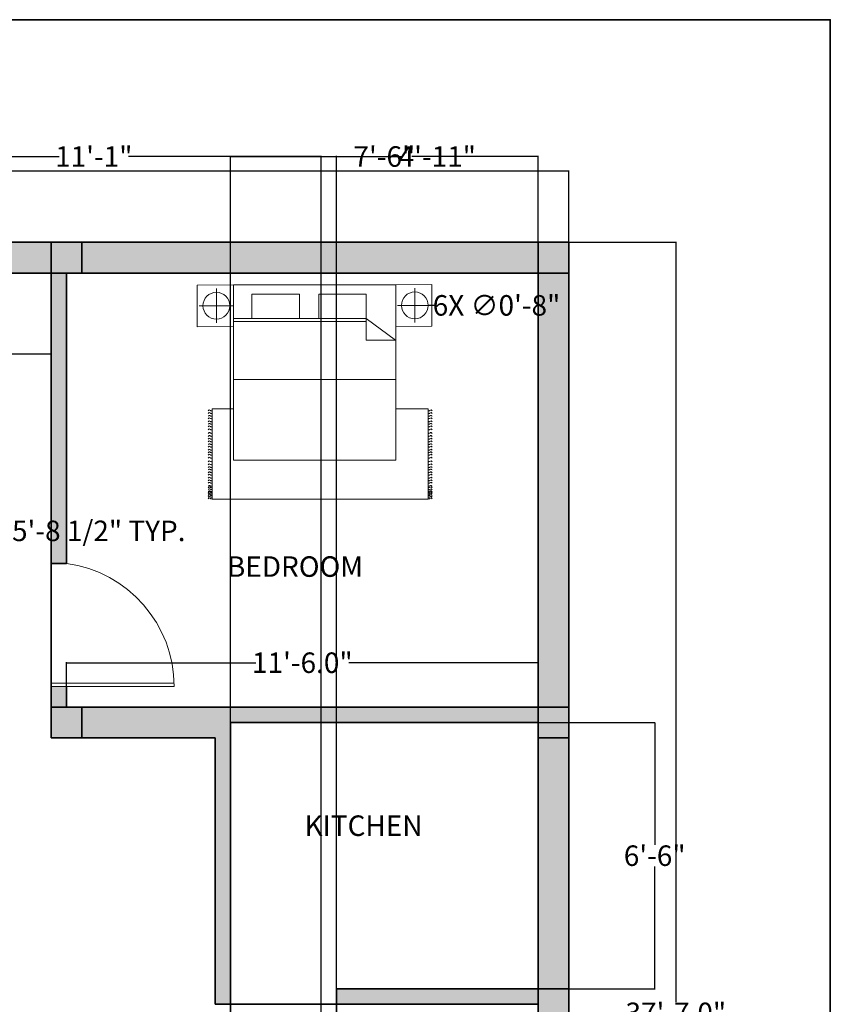
# Model space of a CAD drawing. Units: inches. Extents: x 74 to 548, y 68 to 649.
# Tile 6 of 6: x 311 to 548, y 361 to 649. Entities that reach past the tile are written whole.
import ezdxf

# ---------------------------------------------------------------- set-up
doc = ezdxf.new("R2010")
doc.units = ezdxf.units.IN
doc.header["$MEASUREMENT"] = 0
for name, color, linetype, lineweight in [('A-ANNO-DIMS', 2, 'Continuous', 18), ('A-ANNO-TTLB', 7, 'Continuous', 35), ('A-AREA-IDEN', 7, 'Continuous', 25), ('A-COLS', 7, 'Continuous', 35), ('A-DOOR', 3, 'Continuous', 18), ('A-FURN', 8, 'Continuous', 18), ('A-WALL', 7, 'Continuous', 35)]:
    doc.layers.add(name, color=color, linetype=linetype, lineweight=lineweight)
doc.layers.add('A-COLS-PATT', color=11, linetype='Continuous', lineweight=13, true_color=0xf27172)
doc.layers.add('A-WALL-PATT', color=7, linetype='Continuous', lineweight=13, true_color=0xffffff)
doc.styles.get("Standard").update_dxf_attribs({"font": 'arial.ttf'})
doc.dimstyles.get("Standard").update_dxf_attribs({"dimtxt": 6, "dimasz": 0.18, "dimexe": 0.18, "dimexo": 0.0625, "dimgap": 0.09, "dimtad": 0, "dimtih": 1, "dimtoh": 1, "dimdec": 1, "dimzin": 0, "dimdsep": 46, "dimlunit": 3, "dimtxsty": 'Standard', "dimcen": 0.09, "dimadec": 0, "dimazin": 0, "dimtfac": 1, "dimtdec": 1, "dimtofl": 0, "dimtmove": 0, "dimatfit": 3, "dimfxl": 1, "dimtolj": 1, "dimtzin": 0, "dimarcsym": 0})

# ---------------------------------------------------------------- blocks, each defined once
blk = doc.blocks.new('*D3')
at = {"layer": 'A-ANNO-DIMS', "color": 0, "lineweight": -2, "transparency": 16777216}
for p, q in [((114.96, 584.31), (114.96, 605.21)), ((471.96, 584.31), (471.96, 605.21)), ((115.14, 605.03), (279.52, 605.03)), ((471.78, 605.03), (307.4, 605.03))]:
    blk.add_line(p, q, dxfattribs=at)
at = {"layer": 'A-ANNO-DIMS', "color": 0, "transparency": 16777216}
for points in [[(115.14, 605.06), (115.14, 605), (114.96, 605.03)], [(471.78, 605.06), (471.78, 605), (471.96, 605.03)]]:
    blk.add_solid(points, dxfattribs=at)
at = {"layer": 'Defpoints', "color": 0, "transparency": 16777216}
for p in [(471.96, 605.03), (114.96, 584.24), (471.96, 584.24)]:
    blk.add_point(p, dxfattribs=at)
at = {"layer": 'A-ANNO-DIMS', "color": 0, "transparency": 16777216, "insert": (293.46, 605.03), "char_height": 6, "attachment_point": 5}
blk.add_mtext('\\A1;29\'-9.0"', dxfattribs=at)
blk = doc.blocks.new('*D4')
at = {"layer": 'A-ANNO-DIMS', "color": 0, "lineweight": -2, "transparency": 16777216}
for p, q in [((472.02, 584.24), (503.43, 584.24)), ((503.25, 584.06), (503.25, 361.9)), ((503.25, 133.42), (503.25, 355.59)), ((472.02, 133.24), (503.43, 133.24))]:
    blk.add_line(p, q, dxfattribs=at)
at = {"layer": 'A-ANNO-DIMS', "color": 0, "transparency": 16777216}
for points in [[(503.22, 584.06), (503.28, 584.06), (503.25, 584.24)], [(503.22, 133.42), (503.28, 133.42), (503.25, 133.24)]]:
    blk.add_solid(points, dxfattribs=at)
at = {"layer": 'Defpoints', "color": 0, "transparency": 16777216}
for p in [(471.96, 584.24), (471.96, 133.24), (503.25, 133.24)]:
    blk.add_point(p, dxfattribs=at)
at = {"layer": 'A-ANNO-DIMS', "color": 0, "transparency": 16777216, "insert": (503.25, 358.74), "char_height": 6, "attachment_point": 5}
blk.add_mtext('\\A1;37\'-7.0"', dxfattribs=at)
blk = doc.blocks.new('*D5')
at = {"layer": 'A-ANNO-DIMS', "color": 0, "lineweight": -2, "transparency": 16777216}
for p, q in [((266.46, 561.7), (266.46, 551.37)), ((320.46, 559.19), (320.46, 551.37)), ((266.64, 551.55), (281.78, 551.55)), ((320.28, 551.55), (305.14, 551.55))]:
    blk.add_line(p, q, dxfattribs=at)
at = {"layer": 'A-ANNO-DIMS', "color": 0, "transparency": 16777216}
for points in [[(266.64, 551.58), (266.64, 551.52), (266.46, 551.55)], [(320.28, 551.58), (320.28, 551.52), (320.46, 551.55)]]:
    blk.add_solid(points, dxfattribs=at)
at = {"layer": 'Defpoints', "color": 0, "transparency": 16777216}
for p in [(266.46, 561.76), (320.46, 559.25), (320.46, 551.55)]:
    blk.add_point(p, dxfattribs=at)
at = {"layer": 'A-ANNO-DIMS', "color": 0, "transparency": 16777216, "insert": (293.46, 551.55), "char_height": 6, "attachment_point": 5}
blk.add_mtext('\\A1;4\'-6.0"', dxfattribs=at)
blk = doc.blocks.new('*D7')
at = {"layer": 'A-ANNO-DIMS', "color": 0, "lineweight": -2, "transparency": 16777216}
for p, q in [((324.96, 451.31), (324.96, 461.39)), ((325.14, 461.21), (380.35, 461.21)), ((462.78, 461.21), (407.57, 461.21)), ((462.96, 451.31), (462.96, 461.39))]:
    blk.add_line(p, q, dxfattribs=at)
at = {"layer": 'A-ANNO-DIMS', "color": 0, "transparency": 16777216}
for points in [[(325.14, 461.24), (325.14, 461.18), (324.96, 461.21)], [(462.78, 461.24), (462.78, 461.18), (462.96, 461.21)]]:
    blk.add_solid(points, dxfattribs=at)
at = {"layer": 'Defpoints', "color": 0, "transparency": 16777216}
for p in [(462.96, 461.21), (324.96, 451.24), (462.96, 451.24)]:
    blk.add_point(p, dxfattribs=at)
at = {"layer": 'A-ANNO-DIMS', "color": 0, "transparency": 16777216, "insert": (393.96, 461.21), "char_height": 6, "attachment_point": 5}
blk.add_mtext('\\A1;11\'-6.0"', dxfattribs=at)
blk = doc.blocks.new('BED-DOUBLE-NIGHTSTANDS')
for p, q in [((-5.03, -1.07), (-5.03, -11.12)), ((53.03, -0.96), (53.03, -11.02)), ((0, -6.09), (-10.05, -6.09)), ((58.05, -5.99), (48, -5.99)), ((38.76, -9.86), (0, -9.86)), ((38.82, -10.68), (0, -10.68)), ((38.76, -9.86), (47.38, -16.22)), ((38.82, -9.86), (38.82, -16.22)), ((38.82, -16.22), (47.38, -16.22)), ((47.43, -27.72), (0, -27.72)), ((-6.27, -62.68), (-6.27, -36.31)), ((-6.27, -36.31), (0.03, -36.31)), ((47.43, -36.31), (56.97, -36.31)), ((56.97, -36.31), (56.97, -62.68)), ((56.97, -62.68), (-6.27, -62.68))]:
    blk.add_line(p, q)
for points in [[(-10.63, -12.29), (0, -12.19), (0, 0), (-10.63, -0.1)], [(47.43, 0), (47.43, -51.32), (0, -51.32), (0, 0)], [(47.43, -12.19), (58.05, -12.08), (58.05, 0.1), (47.43, 0)], [(19.25, -2.7), (19.25, -9.86), (5.36, -9.86), (5.36, -2.7)], [(38.82, -2.7), (38.82, -9.86), (24.92, -9.86), (24.92, -2.7)]]:
    blk.add_lwpolyline(points, close=True)
for centre in [(-5.03, -6.09), (53.03, -5.99)]:
    blk.add_circle(centre, 3.92)
for points, knots in [([(-7.4, -36.85), (-7.3, -36.72), (-7.11, -36.49), (-6.77, -36.72), (-6.49, -36.9), (-6.34, -36.79), (-6.27, -36.74)], [0, 0, 0, 0, 0.400747, 0.791423, 1.067667, 1.29709, 1.29709, 1.29709, 1.29709]), ([(-7.4, -37.62), (-7.3, -37.5), (-7.11, -37.26), (-6.77, -37.5), (-6.49, -37.68), (-6.34, -37.57), (-6.27, -37.52)], [0, 0, 0, 0, 0.400747, 0.791423, 1.067667, 1.29709, 1.29709, 1.29709, 1.29709]), ([(58.08, -36.85), (57.99, -36.72), (57.8, -36.49), (57.45, -36.72), (57.17, -36.9), (57.02, -36.79), (56.96, -36.74)], [0, 0, 0, 0, 0.400747, 0.791423, 1.067667, 1.29709, 1.29709, 1.29709, 1.29709]), ([(58.08, -37.62), (57.99, -37.5), (57.8, -37.26), (57.45, -37.5), (57.17, -37.68), (57.02, -37.57), (56.96, -37.52)], [0, 0, 0, 0, 0.400747, 0.791423, 1.067667, 1.29709, 1.29709, 1.29709, 1.29709]), ([(-7.4, -38.44), (-7.3, -38.32), (-7.11, -38.08), (-6.77, -38.32), (-6.49, -38.49), (-6.34, -38.39), (-6.27, -38.34)], [0, 0, 0, 0, 0.400747, 0.791423, 1.067667, 1.29709, 1.29709, 1.29709, 1.29709]), ([(-7.4, -39.17), (-7.3, -39.05), (-7.11, -38.81), (-6.77, -39.05), (-6.49, -39.22), (-6.34, -39.11), (-6.27, -39.07)], [0, 0, 0, 0, 0.400747, 0.791423, 1.067667, 1.29709, 1.29709, 1.29709, 1.29709]), ([(-7.4, -40.05), (-7.3, -39.93), (-7.11, -39.69), (-6.77, -39.93), (-6.49, -40.1), (-6.34, -40), (-6.27, -39.95)], [0, 0, 0, 0, 0.400747, 0.791423, 1.067667, 1.29709, 1.29709, 1.29709, 1.29709]), ([(58.08, -38.44), (57.99, -38.32), (57.8, -38.08), (57.45, -38.32), (57.17, -38.49), (57.02, -38.39), (56.96, -38.34)], [0, 0, 0, 0, 0.400747, 0.791423, 1.067667, 1.29709, 1.29709, 1.29709, 1.29709]), ([(58.08, -39.17), (57.99, -39.05), (57.8, -38.81), (57.45, -39.05), (57.17, -39.22), (57.02, -39.11), (56.96, -39.07)], [0, 0, 0, 0, 0.400747, 0.791423, 1.067667, 1.29709, 1.29709, 1.29709, 1.29709]), ([(58.08, -40.05), (57.99, -39.93), (57.8, -39.69), (57.45, -39.93), (57.17, -40.1), (57.02, -40), (56.96, -39.95)], [0, 0, 0, 0, 0.400747, 0.791423, 1.067667, 1.29709, 1.29709, 1.29709, 1.29709]), ([(-7.4, -40.8), (-7.3, -40.68), (-7.11, -40.44), (-6.77, -40.68), (-6.49, -40.85), (-6.34, -40.75), (-6.27, -40.7)], [0, 0, 0, 0, 0.400747, 0.791423, 1.067667, 1.29709, 1.29709, 1.29709, 1.29709]), ([(-7.4, -41.53), (-7.3, -41.41), (-7.11, -41.17), (-6.77, -41.41), (-6.49, -41.58), (-6.34, -41.48), (-6.27, -41.43)], [0, 0, 0, 0, 0.400747, 0.791423, 1.067667, 1.29709, 1.29709, 1.29709, 1.29709]), ([(-7.4, -42.41), (-7.3, -42.29), (-7.11, -42.05), (-6.77, -42.29), (-6.49, -42.46), (-6.34, -42.36), (-6.27, -42.31)], [0, 0, 0, 0, 0.400747, 0.791423, 1.067667, 1.29709, 1.29709, 1.29709, 1.29709]), ([(-7.4, -43.45), (-7.3, -43.33), (-7.11, -43.09), (-6.77, -43.33), (-6.49, -43.5), (-6.34, -43.39), (-6.27, -43.35)], [0, 0, 0, 0, 0.400747, 0.791423, 1.067667, 1.29709, 1.29709, 1.29709, 1.29709]), ([(58.08, -40.8), (57.99, -40.68), (57.8, -40.44), (57.45, -40.68), (57.17, -40.85), (57.02, -40.75), (56.96, -40.7)], [0, 0, 0, 0, 0.400747, 0.791423, 1.067667, 1.29709, 1.29709, 1.29709, 1.29709]), ([(58.08, -41.53), (57.99, -41.41), (57.8, -41.17), (57.45, -41.41), (57.17, -41.58), (57.02, -41.48), (56.96, -41.43)], [0, 0, 0, 0, 0.400747, 0.791423, 1.067667, 1.29709, 1.29709, 1.29709, 1.29709]), ([(58.08, -42.41), (57.99, -42.29), (57.8, -42.05), (57.45, -42.29), (57.17, -42.46), (57.02, -42.36), (56.96, -42.31)], [0, 0, 0, 0, 0.400747, 0.791423, 1.067667, 1.29709, 1.29709, 1.29709, 1.29709]), ([(58.08, -43.45), (57.99, -43.33), (57.8, -43.09), (57.45, -43.33), (57.17, -43.5), (57.02, -43.39), (56.96, -43.35)], [0, 0, 0, 0, 0.400747, 0.791423, 1.067667, 1.29709, 1.29709, 1.29709, 1.29709]), ([(-7.4, -44.33), (-7.3, -44.21), (-7.11, -43.97), (-6.77, -44.21), (-6.49, -44.38), (-6.34, -44.28), (-6.27, -44.23)], [0, 0, 0, 0, 0.400747, 0.791423, 1.067667, 1.29709, 1.29709, 1.29709, 1.29709]), ([(-7.4, -45.15), (-7.3, -45.03), (-7.11, -44.79), (-6.77, -45.03), (-6.49, -45.2), (-6.34, -45.09), (-6.27, -45.05)], [0, 0, 0, 0, 0.400747, 0.791423, 1.067667, 1.29709, 1.29709, 1.29709, 1.29709]), ([(-7.4, -45.92), (-7.3, -45.8), (-7.11, -45.56), (-6.77, -45.8), (-6.49, -45.98), (-6.34, -45.87), (-6.27, -45.82)], [0, 0, 0, 0, 0.400747, 0.791423, 1.067667, 1.29709, 1.29709, 1.29709, 1.29709]), ([(58.08, -44.33), (57.99, -44.21), (57.8, -43.97), (57.45, -44.21), (57.17, -44.38), (57.02, -44.28), (56.96, -44.23)], [0, 0, 0, 0, 0.400747, 0.791423, 1.067667, 1.29709, 1.29709, 1.29709, 1.29709]), ([(58.08, -45.15), (57.99, -45.03), (57.8, -44.79), (57.45, -45.03), (57.17, -45.2), (57.02, -45.09), (56.96, -45.05)], [0, 0, 0, 0, 0.400747, 0.791423, 1.067667, 1.29709, 1.29709, 1.29709, 1.29709]), ([(58.08, -45.92), (57.99, -45.8), (57.8, -45.56), (57.45, -45.8), (57.17, -45.98), (57.02, -45.87), (56.96, -45.82)], [0, 0, 0, 0, 0.400747, 0.791423, 1.067667, 1.29709, 1.29709, 1.29709, 1.29709]), ([(-7.4, -46.74), (-7.3, -46.62), (-7.11, -46.38), (-6.77, -46.62), (-6.49, -46.79), (-6.34, -46.69), (-6.27, -46.64)], [0, 0, 0, 0, 0.400747, 0.791423, 1.067667, 1.29709, 1.29709, 1.29709, 1.29709]), ([(-7.4, -47.47), (-7.3, -47.35), (-7.11, -47.11), (-6.77, -47.35), (-6.49, -47.52), (-6.34, -47.41), (-6.27, -47.37)], [0, 0, 0, 0, 0.400747, 0.791423, 1.067667, 1.29709, 1.29709, 1.29709, 1.29709]), ([(-7.4, -48.35), (-7.3, -48.23), (-7.11, -47.99), (-6.77, -48.23), (-6.49, -48.4), (-6.34, -48.3), (-6.27, -48.25)], [0, 0, 0, 0, 0.400747, 0.791423, 1.067667, 1.29709, 1.29709, 1.29709, 1.29709]), ([(-7.4, -49.1), (-7.3, -48.98), (-7.11, -48.74), (-6.77, -48.98), (-6.49, -49.15), (-6.34, -49.05), (-6.27, -49)], [0, 0, 0, 0, 0.400747, 0.791423, 1.067667, 1.29709, 1.29709, 1.29709, 1.29709]), ([(58.08, -46.74), (57.99, -46.62), (57.8, -46.38), (57.45, -46.62), (57.17, -46.79), (57.02, -46.69), (56.96, -46.64)], [0, 0, 0, 0, 0.400747, 0.791423, 1.067667, 1.29709, 1.29709, 1.29709, 1.29709]), ([(58.08, -47.47), (57.99, -47.35), (57.8, -47.11), (57.45, -47.35), (57.17, -47.52), (57.02, -47.41), (56.96, -47.37)], [0, 0, 0, 0, 0.400747, 0.791423, 1.067667, 1.29709, 1.29709, 1.29709, 1.29709]), ([(58.08, -48.35), (57.99, -48.23), (57.8, -47.99), (57.45, -48.23), (57.17, -48.4), (57.02, -48.3), (56.96, -48.25)], [0, 0, 0, 0, 0.400747, 0.791423, 1.067667, 1.29709, 1.29709, 1.29709, 1.29709]), ([(58.08, -49.1), (57.99, -48.98), (57.8, -48.74), (57.45, -48.98), (57.17, -49.15), (57.02, -49.05), (56.96, -49)], [0, 0, 0, 0, 0.400747, 0.791423, 1.067667, 1.29709, 1.29709, 1.29709, 1.29709]), ([(-7.4, -49.83), (-7.3, -49.71), (-7.11, -49.47), (-6.77, -49.71), (-6.49, -49.88), (-6.34, -49.78), (-6.27, -49.73)], [0, 0, 0, 0, 0.400747, 0.791423, 1.067667, 1.29709, 1.29709, 1.29709, 1.29709]), ([(-7.4, -50.71), (-7.3, -50.59), (-7.11, -50.35), (-6.77, -50.59), (-6.49, -50.77), (-6.34, -50.66), (-6.27, -50.61)], [0, 0, 0, 0, 0.400747, 0.791423, 1.067667, 1.29709, 1.29709, 1.29709, 1.29709]), ([(-7.4, -51.75), (-7.3, -51.63), (-7.11, -51.39), (-6.77, -51.63), (-6.49, -51.8), (-6.34, -51.7), (-6.27, -51.65)], [0, 0, 0, 0, 0.400747, 0.791423, 1.067667, 1.29709, 1.29709, 1.29709, 1.29709]), ([(58.08, -49.83), (57.99, -49.71), (57.8, -49.47), (57.45, -49.71), (57.17, -49.88), (57.02, -49.78), (56.96, -49.73)], [0, 0, 0, 0, 0.400747, 0.791423, 1.067667, 1.29709, 1.29709, 1.29709, 1.29709]), ([(58.08, -50.71), (57.99, -50.59), (57.8, -50.35), (57.45, -50.59), (57.17, -50.77), (57.02, -50.66), (56.96, -50.61)], [0, 0, 0, 0, 0.400747, 0.791423, 1.067667, 1.29709, 1.29709, 1.29709, 1.29709]), ([(58.08, -51.75), (57.99, -51.63), (57.8, -51.39), (57.45, -51.63), (57.17, -51.8), (57.02, -51.7), (56.96, -51.65)], [0, 0, 0, 0, 0.400747, 0.791423, 1.067667, 1.29709, 1.29709, 1.29709, 1.29709]), ([(-7.4, -52.63), (-7.3, -52.51), (-7.11, -52.27), (-6.77, -52.51), (-6.49, -52.68), (-6.34, -52.58), (-6.27, -52.53)], [0, 0, 0, 0, 0.400747, 0.791423, 1.067667, 1.29709, 1.29709, 1.29709, 1.29709]), ([(-7.4, -53.45), (-7.3, -53.33), (-7.11, -53.09), (-6.77, -53.33), (-6.49, -53.5), (-6.34, -53.39), (-6.27, -53.35)], [0, 0, 0, 0, 0.400747, 0.791423, 1.067667, 1.29709, 1.29709, 1.29709, 1.29709]), ([(-7.4, -54.14), (-7.3, -54.02), (-7.11, -53.78), (-6.77, -54.02), (-6.49, -54.19), (-6.34, -54.08), (-6.27, -54.04)], [0, 0, 0, 0, 0.400747, 0.791423, 1.067667, 1.29709, 1.29709, 1.29709, 1.29709]), ([(-7.4, -54.95), (-7.3, -54.83), (-7.11, -54.59), (-6.77, -54.83), (-6.49, -55.01), (-6.34, -54.9), (-6.27, -54.85)], [0, 0, 0, 0, 0.400747, 0.791423, 1.067667, 1.29709, 1.29709, 1.29709, 1.29709]), ([(58.08, -52.63), (57.99, -52.51), (57.8, -52.27), (57.45, -52.51), (57.17, -52.68), (57.02, -52.58), (56.96, -52.53)], [0, 0, 0, 0, 0.400747, 0.791423, 1.067667, 1.29709, 1.29709, 1.29709, 1.29709]), ([(58.08, -53.45), (57.99, -53.33), (57.8, -53.09), (57.45, -53.33), (57.17, -53.5), (57.02, -53.39), (56.96, -53.35)], [0, 0, 0, 0, 0.400747, 0.791423, 1.067667, 1.29709, 1.29709, 1.29709, 1.29709]), ([(58.08, -54.14), (57.99, -54.02), (57.8, -53.78), (57.45, -54.02), (57.17, -54.19), (57.02, -54.08), (56.96, -54.04)], [0, 0, 0, 0, 0.400747, 0.791423, 1.067667, 1.29709, 1.29709, 1.29709, 1.29709]), ([(58.08, -54.95), (57.99, -54.83), (57.8, -54.59), (57.45, -54.83), (57.17, -55.01), (57.02, -54.9), (56.96, -54.85)], [0, 0, 0, 0, 0.400747, 0.791423, 1.067667, 1.29709, 1.29709, 1.29709, 1.29709]), ([(-7.4, -55.68), (-7.3, -55.56), (-7.11, -55.32), (-6.77, -55.56), (-6.49, -55.73), (-6.34, -55.63), (-6.27, -55.58)], [0, 0, 0, 0, 0.400747, 0.791423, 1.067667, 1.29709, 1.29709, 1.29709, 1.29709]), ([(-7.4, -56.56), (-7.3, -56.44), (-7.11, -56.2), (-6.77, -56.44), (-6.49, -56.62), (-6.34, -56.51), (-6.27, -56.46)], [0, 0, 0, 0, 0.400747, 0.791423, 1.067667, 1.29709, 1.29709, 1.29709, 1.29709]), ([(-7.4, -57.32), (-7.3, -57.2), (-7.11, -56.96), (-6.77, -57.2), (-6.49, -57.37), (-6.34, -57.26), (-6.27, -57.21)], [0, 0, 0, 0, 0.400747, 0.791423, 1.067667, 1.29709, 1.29709, 1.29709, 1.29709]), ([(58.08, -55.68), (57.99, -55.56), (57.8, -55.32), (57.45, -55.56), (57.17, -55.73), (57.02, -55.63), (56.96, -55.58)], [0, 0, 0, 0, 0.400747, 0.791423, 1.067667, 1.29709, 1.29709, 1.29709, 1.29709]), ([(58.08, -56.56), (57.99, -56.44), (57.8, -56.2), (57.45, -56.44), (57.17, -56.62), (57.02, -56.51), (56.96, -56.46)], [0, 0, 0, 0, 0.400747, 0.791423, 1.067667, 1.29709, 1.29709, 1.29709, 1.29709]), ([(58.08, -57.32), (57.99, -57.2), (57.8, -56.96), (57.45, -57.2), (57.17, -57.37), (57.02, -57.26), (56.96, -57.21)], [0, 0, 0, 0, 0.400747, 0.791423, 1.067667, 1.29709, 1.29709, 1.29709, 1.29709]), ([(-7.4, -58.04), (-7.3, -57.92), (-7.11, -57.68), (-6.77, -57.92), (-6.49, -58.1), (-6.34, -57.99), (-6.27, -57.94)], [0, 0, 0, 0, 0.400747, 0.791423, 1.067667, 1.29709, 1.29709, 1.29709, 1.29709]), ([(-7.4, -58.93), (-7.3, -58.81), (-7.11, -58.57), (-6.77, -58.81), (-6.49, -58.98), (-6.34, -58.87), (-6.27, -58.82)], [0, 0, 0, 0, 0.400747, 0.791423, 1.067667, 1.29709, 1.29709, 1.29709, 1.29709]), ([(-7.4, -59.36), (-7.3, -59.23), (-7.11, -58.98), (-6.77, -59.24), (-6.49, -59.41), (-6.34, -59.3), (-6.27, -59.25)], [0, 0, 0, 0, 0.407265, 0.802015, 1.07826, 1.307683, 1.307683, 1.307683, 1.307683]), ([(-7.4, -59.92), (-7.3, -59.8), (-7.11, -59.56), (-6.77, -59.8), (-6.49, -59.97), (-6.34, -59.87), (-6.27, -59.82)], [0, 0, 0, 0, 0.400747, 0.791423, 1.067667, 1.29709, 1.29709, 1.29709, 1.29709]), ([(-7.4, -60.5), (-7.3, -60.38), (-7.11, -60.14), (-6.77, -60.38), (-6.49, -60.55), (-6.34, -60.44), (-6.27, -60.39)], [0, 0, 0, 0, 0.400747, 0.791423, 1.067667, 1.29709, 1.29709, 1.29709, 1.29709]), ([(58.08, -58.04), (57.99, -57.92), (57.8, -57.68), (57.45, -57.92), (57.18, -58.09), (57.03, -57.99), (56.97, -57.95)], [0, 0, 0, 0, 0.400747, 0.791423, 1.067667, 1.283686, 1.283686, 1.283686, 1.283686]), ([(58.08, -58.93), (57.99, -58.81), (57.8, -58.57), (57.45, -58.81), (57.18, -58.98), (57.03, -58.88), (56.97, -58.83)], [0, 0, 0, 0, 0.400747, 0.791423, 1.067667, 1.283686, 1.283686, 1.283686, 1.283686]), ([(58.08, -59.36), (57.99, -59.23), (57.8, -58.99), (57.45, -59.24), (57.18, -59.41), (57.03, -59.31), (56.97, -59.26)], [0, 0, 0, 0, 0.402903, 0.794912, 1.071156, 1.287177, 1.287177, 1.287177, 1.287177]), ([(58.08, -59.95), (57.99, -59.83), (57.8, -59.59), (57.45, -59.83), (57.18, -60), (57.03, -59.9), (56.97, -59.86)], [0, 0, 0, 0, 0.400747, 0.791423, 1.067667, 1.283686, 1.283686, 1.283686, 1.283686]), ([(58.08, -60.52), (57.99, -60.4), (57.8, -60.16), (57.45, -60.4), (57.18, -60.57), (57.03, -60.47), (56.97, -60.43)], [0, 0, 0, 0, 0.400747, 0.791423, 1.067667, 1.283686, 1.283686, 1.283686, 1.283686]), ([(-7.4, -60.81), (-7.3, -60.68), (-7.11, -60.44), (-6.77, -60.68), (-6.49, -60.86), (-6.34, -60.75), (-6.27, -60.7)], [0, 0, 0, 0, 0.400747, 0.791423, 1.067667, 1.29709, 1.29709, 1.29709, 1.29709]), ([(-7.4, -61.22), (-7.3, -61.1), (-7.11, -60.86), (-6.77, -61.1), (-6.49, -61.28), (-6.34, -61.17), (-6.27, -61.12)], [0, 0, 0, 0, 0.400747, 0.791423, 1.067667, 1.29709, 1.29709, 1.29709, 1.29709]), ([(-7.4, -61.62), (-7.3, -61.5), (-7.11, -61.26), (-6.77, -61.5), (-6.49, -61.67), (-6.34, -61.57), (-6.27, -61.52)], [0, 0, 0, 0, 0.400747, 0.791423, 1.067667, 1.29709, 1.29709, 1.29709, 1.29709]), ([(-7.4, -62.11), (-7.3, -61.99), (-7.11, -61.75), (-6.77, -61.99), (-6.49, -62.16), (-6.34, -62.05), (-6.27, -62)], [0, 0, 0, 0, 0.400747, 0.791423, 1.067667, 1.29709, 1.29709, 1.29709, 1.29709]), ([(-7.4, -62.61), (-7.3, -62.49), (-7.11, -62.25), (-6.77, -62.49), (-6.49, -62.66), (-6.34, -62.55), (-6.27, -62.51)], [0, 0, 0, 0, 0.400747, 0.791423, 1.067667, 1.29709, 1.29709, 1.29709, 1.29709]), ([(58.08, -61.25), (57.99, -61.13), (57.8, -60.89), (57.45, -61.13), (57.17, -61.3), (57.02, -61.2), (56.96, -61.15)], [0, 0, 0, 0, 0.400747, 0.791423, 1.067667, 1.29709, 1.29709, 1.29709, 1.29709]), ([(58.08, -61.65), (57.99, -61.53), (57.8, -61.29), (57.45, -61.53), (57.17, -61.7), (57.02, -61.6), (56.96, -61.55)], [0, 0, 0, 0, 0.400747, 0.791423, 1.067667, 1.29709, 1.29709, 1.29709, 1.29709]), ([(58.08, -62.13), (57.99, -62.01), (57.8, -61.77), (57.45, -62.01), (57.17, -62.19), (57.02, -62.08), (56.96, -62.03)], [0, 0, 0, 0, 0.400747, 0.791423, 1.067667, 1.29709, 1.29709, 1.29709, 1.29709]), ([(58.08, -62.61), (57.99, -62.49), (57.8, -62.25), (57.45, -62.49), (57.17, -62.66), (57.02, -62.55), (56.96, -62.51)], [0, 0, 0, 0, 0.400747, 0.791423, 1.067667, 1.29709, 1.29709, 1.29709, 1.29709]), ([(58.08, -60.83), (57.99, -60.71), (57.8, -60.47), (57.45, -60.71), (57.18, -60.88), (57.03, -60.78), (56.97, -60.74)], [0, 0, 0, 0, 0.400747, 0.791423, 1.067667, 1.283686, 1.283686, 1.283686, 1.283686])]:
    blk.add_open_spline(points, degree=3, knots=knots)
blk = doc.blocks.new('DOOR-SWING-36IN')
for p, q in [((0, 0), (0, 36)), ((-36, 1), (0, 1)), ((0, 0), (-36, 0))]:
    blk.add_line(p, q)
blk.add_arc((0.32, 0), 36.32, 97.6281, 180)
blk = doc.blocks.new('*D12')
at = {"layer": 'A-ANNO-DIMS', "color": 0, "lineweight": -2, "transparency": 16777216}
for p, q in [((153.88, 510.03), (153.88, 499.61)), ((222.59, 510.03), (222.59, 499.61)), ((154.06, 499.79), (222.41, 499.79)), ((222.59, 499.79), (222.77, 499.79))]:
    blk.add_line(p, q, dxfattribs=at)
at = {"layer": 'A-ANNO-DIMS', "color": 0, "transparency": 16777216}
for points in [[(154.06, 499.82), (154.06, 499.76), (153.88, 499.79)], [(222.41, 499.82), (222.41, 499.76), (222.59, 499.79)]]:
    blk.add_solid(points, dxfattribs=at)
at = {"layer": 'Defpoints', "color": 0, "transparency": 16777216}
for p in [(153.88, 510.09), (222.59, 510.09), (222.59, 499.79)]:
    blk.add_point(p, dxfattribs=at)
at = {"layer": 'A-ANNO-DIMS', "color": 0, "transparency": 16777216, "insert": (292.95, 499.79), "char_height": 6, "attachment_point": 5}
blk.add_mtext('\\A1;BED & NIGHTSTANDS 5\'-8 1/2" TYP.', dxfattribs=at)
blk = doc.blocks.new('*D21')
at = {"layer": 'A-ANNO-DIMS', "color": 0, "lineweight": -2, "transparency": 16777216}
for p, q in [((372.96, 361.31), (372.96, 609.52)), ((373.14, 609.34), (409.92, 609.34)), ((462.78, 609.34), (426, 609.34)), ((462.96, 356.81), (462.96, 609.52))]:
    blk.add_line(p, q, dxfattribs=at)
at = {"layer": 'A-ANNO-DIMS', "color": 0, "transparency": 16777216}
for points in [[(373.14, 609.37), (373.14, 609.31), (372.96, 609.34)], [(462.78, 609.37), (462.78, 609.31), (462.96, 609.34)]]:
    blk.add_solid(points, dxfattribs=at)
at = {"layer": 'Defpoints', "color": 0, "transparency": 16777216}
for p in [(462.96, 609.34), (372.96, 361.24), (462.96, 356.74)]:
    blk.add_point(p, dxfattribs=at)
at = {"layer": 'A-ANNO-DIMS', "color": 0, "transparency": 16777216, "insert": (417.96, 609.34), "char_height": 6, "attachment_point": 5}
blk.add_mtext('\\A1;7\'-6"', dxfattribs=at)
blk = doc.blocks.new('*D22')
at = {"layer": 'A-ANNO-DIMS', "color": 0, "lineweight": -2, "transparency": 16777216}
for p, q in [((463.02, 443.74), (497.24, 443.74)), ((497.06, 443.56), (497.06, 407.9)), ((497.06, 365.92), (497.06, 401.59)), ((403.99, 365.74), (497.24, 365.74))]:
    blk.add_line(p, q, dxfattribs=at)
at = {"layer": 'A-ANNO-DIMS', "color": 0, "transparency": 16777216}
for points in [[(497.03, 443.56), (497.09, 443.56), (497.06, 443.74)], [(497.03, 365.92), (497.09, 365.92), (497.06, 365.74)]]:
    blk.add_solid(points, dxfattribs=at)
at = {"layer": 'Defpoints', "color": 0, "transparency": 16777216}
for p in [(462.96, 443.74), (497.06, 443.74), (403.93, 365.74)]:
    blk.add_point(p, dxfattribs=at)
at = {"layer": 'A-ANNO-DIMS', "color": 0, "transparency": 16777216, "insert": (497.06, 404.74), "char_height": 6, "attachment_point": 5}
blk.add_mtext('\\A1;6\'-6"', dxfattribs=at)
blk = doc.blocks.new('*D24')
at = {"layer": 'A-ANNO-DIMS', "color": 0, "lineweight": -2, "transparency": 16777216}
for p, q in [((403.93, 223.31), (403.93, 609.52)), ((404.11, 609.34), (422.93, 609.34)), ((462.78, 609.34), (443.96, 609.34)), ((462.96, 133.31), (462.96, 609.52))]:
    blk.add_line(p, q, dxfattribs=at)
at = {"layer": 'A-ANNO-DIMS', "color": 0, "transparency": 16777216}
for points in [[(404.11, 609.37), (404.11, 609.31), (403.93, 609.34)], [(462.78, 609.37), (462.78, 609.31), (462.96, 609.34)]]:
    blk.add_solid(points, dxfattribs=at)
at = {"layer": 'Defpoints', "color": 0, "transparency": 16777216}
for p in [(462.96, 609.34), (403.93, 223.24), (462.96, 133.24)]:
    blk.add_point(p, dxfattribs=at)
at = {"layer": 'A-ANNO-DIMS', "color": 0, "transparency": 16777216, "insert": (433.44, 609.34), "char_height": 6, "attachment_point": 5}
blk.add_mtext('\\A1;4\'-11"', dxfattribs=at)
blk = doc.blocks.new('*D26')
at = {"layer": 'A-ANNO-DIMS', "color": 0, "lineweight": -2, "transparency": 16777216}
for p, q in [((372.96, 142.31), (372.96, 609.52)), ((373.14, 609.34), (409.92, 609.34)), ((462.78, 609.34), (426, 609.34)), ((462.96, 133.31), (462.96, 609.52))]:
    blk.add_line(p, q, dxfattribs=at)
at = {"layer": 'A-ANNO-DIMS', "color": 0, "transparency": 16777216}
for points in [[(373.14, 609.37), (373.14, 609.31), (372.96, 609.34)], [(462.78, 609.37), (462.78, 609.31), (462.96, 609.34)]]:
    blk.add_solid(points, dxfattribs=at)
at = {"layer": 'Defpoints', "color": 0, "transparency": 16777216}
for p in [(462.96, 609.34), (372.96, 142.24), (462.96, 133.24)]:
    blk.add_point(p, dxfattribs=at)
at = {"layer": 'A-ANNO-DIMS', "color": 0, "transparency": 16777216, "insert": (417.96, 609.34), "char_height": 6, "attachment_point": 5}
blk.add_mtext('\\A1;7\'-6"', dxfattribs=at)
blk = doc.blocks.new('*D37')
at = {"layer": 'A-ANNO-DIMS', "color": 0, "lineweight": -2, "transparency": 16777216}
for p, q in [((266.46, 297.87), (266.46, 609.52)), ((266.64, 609.34), (322.83, 609.34)), ((399.25, 609.34), (343.06, 609.34)), ((399.43, 299.06), (399.43, 609.52))]:
    blk.add_line(p, q, dxfattribs=at)
at = {"layer": 'A-ANNO-DIMS', "color": 0, "transparency": 16777216}
for points in [[(266.64, 609.37), (266.64, 609.31), (266.46, 609.34)], [(399.25, 609.37), (399.25, 609.31), (399.43, 609.34)]]:
    blk.add_solid(points, dxfattribs=at)
at = {"layer": 'Defpoints', "color": 0, "transparency": 16777216}
for p in [(399.43, 609.34), (266.46, 297.81), (399.43, 298.99)]:
    blk.add_point(p, dxfattribs=at)
at = {"layer": 'A-ANNO-DIMS', "color": 0, "transparency": 16777216, "insert": (332.94, 609.34), "char_height": 6, "attachment_point": 5}
blk.add_mtext('\\A1;11\'-1"', dxfattribs=at)
blk = doc.blocks.new('*D39')
at = {"layer": 'A-ANNO-DIMS', "color": 0, "lineweight": -2, "transparency": 16777216}
for p, q in [((403.93, 365.68), (403.93, 87.96)), ((372.96, 361.18), (372.96, 87.96)), ((373.14, 88.14), (380.33, 88.14)), ((403.75, 88.14), (396.56, 88.14))]:
    blk.add_line(p, q, dxfattribs=at)
at = {"layer": 'A-ANNO-DIMS', "color": 0, "transparency": 16777216}
for points in [[(373.14, 88.17), (373.14, 88.11), (372.96, 88.14)], [(403.75, 88.17), (403.75, 88.11), (403.93, 88.14)]]:
    blk.add_solid(points, dxfattribs=at)
at = {"layer": 'Defpoints', "color": 0, "transparency": 16777216}
for p in [(403.93, 365.74), (372.96, 361.24), (403.93, 88.14)]:
    blk.add_point(p, dxfattribs=at)
at = {"layer": 'A-ANNO-DIMS', "color": 0, "transparency": 16777216, "insert": (388.44, 88.14), "char_height": 6, "attachment_point": 5}
blk.add_mtext('\\A1;2\'-7"', dxfattribs=at)
blk = doc.blocks.new('*D46')
at = {"layer": 'A-ANNO-DIMS', "color": 0, "lineweight": -2, "transparency": 16777216}
for p, q in [((426.78, 565.78), (426.96, 565.78)), ((426.87, 565.69), (426.87, 565.87)), ((433.15, 565.78), (430.97, 565.78))]:
    blk.add_line(p, q, dxfattribs=at)
at = {"layer": 'A-ANNO-DIMS', "color": 0, "transparency": 16777216}
blk.add_solid([(430.97, 565.81), (430.97, 565.75), (430.79, 565.78)], dxfattribs=at)
at = {"layer": 'Defpoints', "color": 0, "transparency": 16777216}
for p in [(422.95, 565.78), (430.79, 565.78)]:
    blk.add_point(p, dxfattribs=at)
at = {"layer": 'A-ANNO-DIMS', "color": 0, "transparency": 16777216, "insert": (450.78, 565.78), "char_height": 6, "attachment_point": 5}
blk.add_mtext('\\A1;6X ∅0\'-8"', dxfattribs=at)

msp = doc.modelspace()

# ---------------------------------------------------------------- hatches: boundary and pattern name
at = {"layer": 'A-COLS-PATT'}
h = msp.add_hatch(color=256, dxfattribs=at)
h.dxf.hatch_style = 1
h.paths.add_polyline_path([(123.96, 584.24), (114.96, 584.24), (114.96, 575.24), (123.96, 575.24)])
h.paths.add_polyline_path([(266.46, 584.24), (257.46, 584.24), (257.46, 575.24), (266.46, 575.24)])
h.paths.add_polyline_path([(329.46, 584.24), (320.46, 584.24), (320.46, 575.24), (329.46, 575.24)])
h.paths.add_polyline_path([(471.96, 584.24), (462.96, 584.24), (462.96, 575.24), (471.96, 575.24)])
h.paths.add_polyline_path([(123.96, 448.24), (114.96, 448.24), (114.96, 439.24), (123.96, 439.24)])
h.paths.add_polyline_path([(266.46, 448.24), (261.96, 448.24), (257.46, 448.24), (257.46, 439.24), (266.46, 439.24)])
h.paths.add_polyline_path([(329.46, 448.24), (320.46, 448.24), (320.46, 439.24), (329.46, 439.24)])
h.paths.add_polyline_path([(471.96, 448.24), (462.96, 448.24), (462.96, 439.24), (471.96, 439.24)])
h.paths.add_polyline_path([(123.96, 365.74), (114.96, 365.74), (114.96, 356.74), (123.96, 356.74)])
h.paths.add_polyline_path([(266.46, 365.74), (257.46, 365.74), (257.46, 356.74), (266.46, 356.74)])
h.paths.add_polyline_path([(123.96, 223.24), (114.96, 223.24), (114.96, 214.24), (123.96, 214.24)])
h.paths.add_polyline_path([(266.46, 223.24), (257.46, 223.24), (257.46, 214.24), (266.46, 214.24)])
h.paths.add_polyline_path([(123.96, 142.24), (114.96, 142.24), (114.96, 133.24), (123.96, 133.24)])
h.paths.add_polyline_path([(263.89, 142.24), (254.89, 142.24), (254.89, 133.24), (263.89, 133.24)])
h.paths.add_polyline_path([(471.96, 142.24), (462.96, 142.24), (462.96, 133.24), (471.96, 133.24)])
h.paths.add_polyline_path([(377.46, 142.24), (368.46, 142.24), (368.46, 133.24), (377.46, 133.24)])
h.paths.add_polyline_path([(377.46, 223.24), (368.46, 223.24), (368.46, 214.24), (377.46, 214.24)])
h.paths.add_polyline_path([(471.96, 223.24), (462.96, 223.24), (462.96, 214.24), (471.96, 214.24)])
h.paths.add_polyline_path([(471.96, 298.99), (462.96, 298.99), (462.96, 289.99), (471.96, 289.99)])
h.paths.add_polyline_path([(471.96, 365.74), (462.96, 365.74), (462.96, 356.74), (471.96, 356.74)])
at = {"layer": 'A-WALL-PATT'}
h = msp.add_hatch(color=256, dxfattribs=at)
h.dxf.hatch_style = 1
h.paths.add_polyline_path([(123.96, 356.74), (114.96, 356.74), (114.96, 223.24), (123.96, 223.24)])
h.paths.add_polyline_path([(123.96, 439.24), (114.96, 439.24), (114.96, 365.74), (123.96, 365.74)])
h.paths.add_polyline_path([(123.96, 575.24), (114.96, 575.24), (114.96, 448.24), (123.96, 448.24)])
h.paths.add_polyline_path([(257.46, 584.24), (123.96, 584.24), (123.96, 575.24), (257.46, 575.24)])
h.paths.add_polyline_path([(266.46, 575.24), (261.96, 575.24), (261.96, 490.24), (266.46, 490.24)])
h.paths.add_polyline_path([(266.46, 454.24), (261.96, 454.24), (261.96, 448.24), (266.46, 448.24)])
h.paths.add_polyline_path([(257.46, 448.24), (187.71, 448.24), (187.71, 443.74), (190.71, 443.74), (190.71, 365.74), (123.96, 365.74), (123.96, 361.24), (257.46, 361.24), (257.46, 365.74), (195.21, 365.74), (195.21, 443.74), (257.46, 443.74)])
h.paths.add_polyline_path([(163.71, 448.24), (123.96, 448.24), (123.96, 443.74), (163.71, 443.74)], flags=17)
h.paths.add_polyline_path([(223.59, 223.24), (220.05, 223.24), (220.05, 216.24), (160.05, 216.24), (160.05, 223.24), (123.96, 223.24), (123.96, 214.24), (159.96, 214.24), (223.59, 214.24)])
h.paths.add_polyline_path([(123.96, 214.24), (114.96, 214.24), (114.96, 142.24), (123.96, 142.24)])
h.paths.add_polyline_path([(254.89, 142.24), (123.96, 142.24), (123.96, 133.24), (254.89, 133.24)])
h.paths.add_polyline_path([(462.96, 142.24), (377.46, 142.24), (377.46, 133.24), (462.96, 133.24)])
h.paths.add_polyline_path([(372.96, 189.24), (368.46, 189.24), (368.46, 142.24), (372.96, 142.24)])
h.paths.add_polyline_path([(471.96, 214.24), (462.96, 214.24), (462.96, 142.24), (471.96, 142.24)])
h.paths.add_polyline_path([(462.96, 223.24), (403.93, 223.24), (403.93, 294.49), (409.93, 294.49), (409.93, 298.99), (403.93, 298.99), (399.43, 298.99), (399.43, 223.24), (377.46, 223.24), (377.46, 214.24), (462.96, 214.24)])
h.paths.add_polyline_path([(368.46, 223.24), (353.46, 223.24), (353.46, 216.24), (305.46, 216.24), (305.46, 223.24), (302.46, 223.24), (302.46, 214.24), (368.46, 214.24)])
h.paths.add_polyline_path([(471.96, 289.99), (462.96, 289.99), (462.96, 223.24), (471.96, 223.24)])
h.paths.add_polyline_path([(462.96, 298.99), (433.93, 298.99), (433.93, 294.49), (462.96, 294.49)], flags=0)
h.paths.add_polyline_path([(471.96, 356.74), (462.96, 356.74), (462.96, 298.99), (471.96, 298.99)])
h.paths.add_polyline_path([(462.96, 365.74), (403.93, 365.74), (403.93, 361.24), (462.96, 361.24)], flags=17)
h.paths.add_polyline_path([(471.96, 439.24), (462.96, 439.24), (462.96, 365.74), (471.96, 365.74)])
h.paths.add_polyline_path([(462.96, 448.24), (329.46, 448.24), (329.46, 439.24), (368.46, 439.24), (368.46, 361.24), (372.96, 361.24), (372.96, 443.74), (462.96, 443.74)])
h.paths.add_polyline_path([(324.96, 454.24), (320.46, 454.24), (320.46, 448.24), (324.96, 448.24)])
h.paths.add_polyline_path([(471.96, 575.24), (462.96, 575.24), (462.96, 448.24), (471.96, 448.24)])
h.paths.add_polyline_path([(462.96, 584.24), (329.46, 584.24), (329.46, 575.24), (462.96, 575.24)])
h.paths.add_polyline_path([(320.46, 584.24), (266.46, 584.24), (266.46, 575.24), (320.46, 575.24)])
h.paths.add_polyline_path([(324.96, 575.24), (320.46, 575.24), (320.46, 490.24), (324.96, 490.24)])
h.paths.add_polyline_path([(266.46, 405.58), (257.46, 405.58), (257.46, 365.74), (266.46, 365.74)])
h.paths.add_polyline_path([(266.46, 356.74), (261.96, 356.74), (261.96, 333.81), (266.46, 333.81)])
h.paths.add_polyline_path([(266.46, 297.81), (261.96, 297.81), (261.96, 223.24), (266.46, 223.24)])

# ---------------------------------------------------------------- linework, layer by layer
at = {"layer": 'A-ANNO-TTLB'}
msp.add_lwpolyline([(82.75, 649.38), (548.44, 649.38), (548.44, 68.13), (82.75, 68.13)], close=True, dxfattribs=at)
at = {"layer": 'A-COLS'}
for p, q in [((320.46, 584.24), (329.46, 584.24)), ((329.46, 584.24), (329.46, 575.24)), ((329.46, 448.24), (320.46, 448.24)), ((329.46, 439.24), (329.46, 448.24)), ((320.46, 439.24), (329.46, 439.24)), ((471.96, 439.24), (462.96, 439.24))]:
    msp.add_line(p, q, dxfattribs=at)
at = {"layer": 'A-DOOR'}
msp.add_line((356.46, 454.24), (320.46, 454.24), dxfattribs=at)
at = {"layer": 'A-WALL'}
for p, q in [((114.96, 584.24), (471.96, 584.24)), ((320.46, 584.24), (320.46, 439.24)), ((462.96, 584.24), (462.96, 133.24)), ((471.96, 584.24), (471.96, 133.24)), ((114.96, 575.24), (471.96, 575.24)), ((324.96, 575.24), (324.96, 490.24)), ((320.46, 490.24), (324.96, 490.24)), ((320.46, 448.24), (320.46, 454.24)), ((324.96, 454.24), (324.96, 448.24)), ((320.46, 448.24), (471.96, 448.24)), ((372.96, 443.74), (372.96, 361.24)), ((372.96, 443.74), (462.96, 443.74)), ((320.46, 439.24), (368.46, 439.24)), ((368.46, 439.24), (368.46, 361.24)), ((403.93, 365.74), (403.93, 361.24)), ((403.93, 361.24), (403.93, 365.74)), ((403.93, 365.74), (471.96, 365.74)), ((368.46, 361.24), (462.96, 361.24))]:
    msp.add_line(p, q, dxfattribs=at)

# ---------------------------------------------------------------- block references
at = {"layer": 'A-DOOR', "extrusion": (0, 0, -1), "zscale": -1}
msp.add_blockref('DOOR-SWING-36IN', (-320.46, 454.24), dxfattribs=at)
at = {"layer": 'A-FURN'}
msp.add_blockref('BED-DOUBLE-NIGHTSTANDS', (373.84, 571.77), dxfattribs=at)

# ---------------------------------------------------------------- texts
at = {"layer": 'A-AREA-IDEN', "char_height": 6, "attachment_point": 1}
for s, width, insert in [('BEDROOM', 52.6995, (371.9, 492.34)), ('KITCHEN', 42.7633, (394.61, 416.51))]:
    msp.add_mtext_dynamic_manual_height_columns(s, width=width, gutter_width=30, heights=[0], dxfattribs=dict(at, insert=insert))

# ---------------------------------------------------------------- dimensions: what is measured, and where the dimension line sits
at = {"layer": 'A-ANNO-DIMS'}
for base, p1, p2, override, picture, middle in [((399.43, 609.34), (266.46, 297.81), (399.43, 298.99), {"dimdec": 1, "dimlfac": 1, "dimrnd": 0, "dimzin": 1, "dimdsep": 46, "dimlunit": 4, "dimfrac": 2}, '*D37', (332.94, 609.34)), ((462.96, 609.34), (372.96, 361.24), (462.96, 356.74), {"dimdec": 1, "dimlfac": 1, "dimrnd": 0, "dimzin": 1, "dimdsep": 46, "dimlunit": 4, "dimfrac": 2}, '*D21', (417.96, 609.34)), ((462.96, 609.34), (372.96, 142.24), (462.96, 133.24), {"dimdec": 1, "dimlfac": 1, "dimrnd": 0, "dimzin": 1, "dimdsep": 46, "dimlunit": 4, "dimfrac": 2}, '*D26', (417.96, 609.34)), ((462.96, 609.34), (403.93, 223.24), (462.96, 133.24), {"dimdec": 1, "dimlfac": 1, "dimrnd": 0, "dimzin": 1, "dimdsep": 46, "dimlunit": 4, "dimfrac": 2}, '*D24', (433.44, 609.34)), ((471.96, 605.03), (114.96, 584.24), (471.96, 584.24), {"dimclrd": 0, "dimclre": 0, "dimclrt": 0}, '*D3', (293.46, 605.03)), ((320.46, 551.55), (266.46, 561.76), (320.46, 559.25), {"dimclrd": 0, "dimclre": 0, "dimclrt": 0}, '*D5', (293.46, 551.55)), ((462.96, 461.21), (324.96, 451.24), (462.96, 451.24), {"dimclrd": 0, "dimclre": 0, "dimclrt": 0}, '*D7', (393.96, 461.21)), ((403.93, 88.14), (372.96, 361.24), (403.93, 365.74), {"dimdec": 1, "dimlfac": 1, "dimrnd": 0, "dimzin": 1, "dimdsep": 46, "dimlunit": 4, "dimfrac": 2}, '*D39', (388.44, 88.14))]:
    dim = msp.add_linear_dim(base=base, p1=p1, p2=p2, dimstyle='Standard', override=override, dxfattribs=at)
    dim.commit()
    dim.dimension.update_dxf_attribs({"geometry": picture, "text_midpoint": middle})
for base, p1, p2, override, picture, middle in [((503.25, 133.24), (471.96, 584.24), (471.96, 133.24), {"dimclrd": 0, "dimclre": 0, "dimclrt": 0}, '*D4', (503.25, 358.74)), ((497.06, 443.74), (403.93, 365.74), (462.96, 443.74), {"dimdec": 1, "dimlfac": 1, "dimrnd": 0, "dimzin": 1, "dimdsep": 46, "dimlunit": 4, "dimfrac": 2}, '*D22', (497.06, 404.74))]:
    dim = msp.add_linear_dim(base=base, p1=p1, p2=p2, angle=90, dimstyle='Standard', override=override, dxfattribs=at)
    dim.commit()
    dim.dimension.update_dxf_attribs({"geometry": picture, "text_midpoint": middle})
dim = msp.add_diameter_dim_2p(p1=(422.95, 565.78), p2=(430.79, 565.78), text='6X <>', dimstyle='Standard', override={"dimdec": 1, "dimlfac": 1, "dimrnd": 0, "dimzin": 1, "dimdsep": 46, "dimlunit": 4, "dimfrac": 2}, dxfattribs=at)
dim.commit()
dim.dimension.update_dxf_attribs({"geometry": '*D46', "text_midpoint": (433.15, 565.78), "dimtype": 163})
dim = msp.add_linear_dim(base=(222.59, 499.79), p1=(153.88, 510.09), p2=(222.59, 510.09), text='BED & NIGHTSTANDS <> TYP.', dimstyle='Standard', override={"dimdec": 1, "dimlfac": 1, "dimrnd": 0, "dimzin": 1, "dimdsep": 46, "dimlunit": 4, "dimfrac": 2}, dxfattribs=at)
dim.commit()
dim.dimension.update_dxf_attribs({"geometry": '*D12', "text_midpoint": (292.95, 499.79)})

doc.saveas('drawing.dxf')
